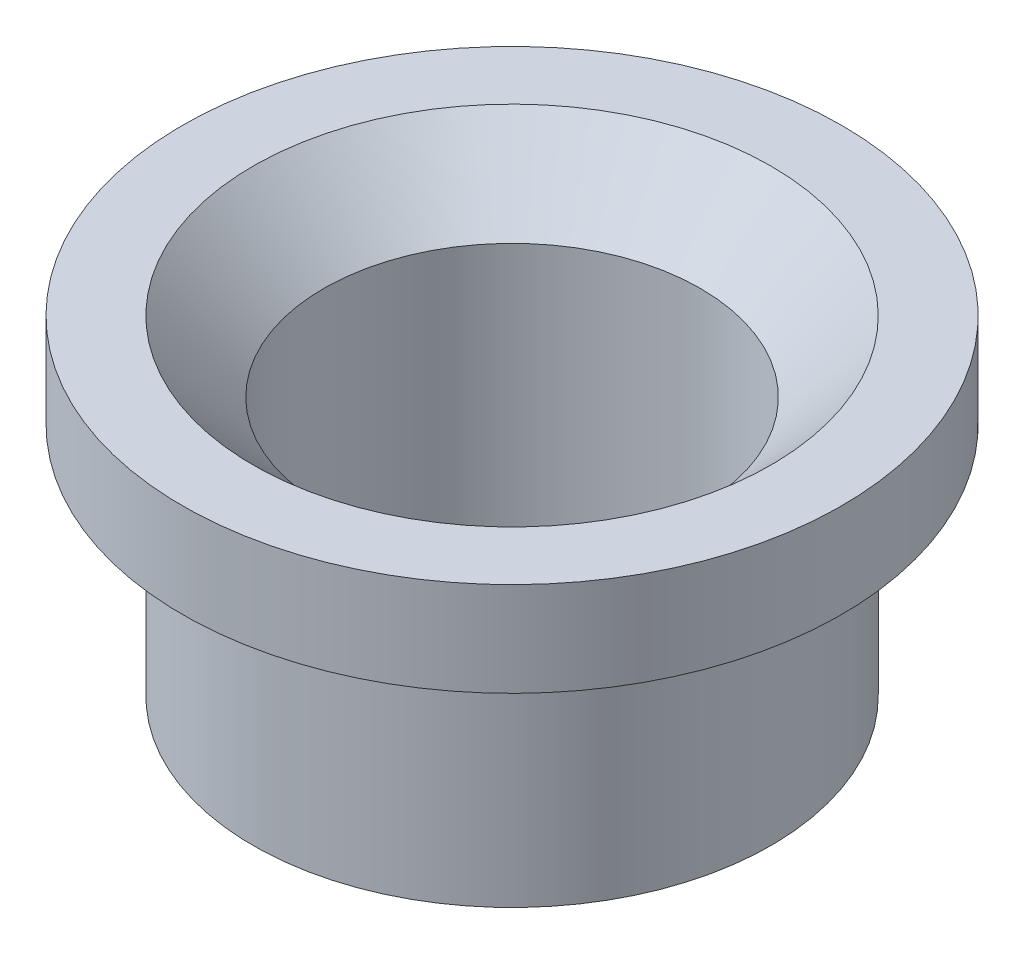
from build123d import *


with BuildPart() as part:
    # Bush Half-Section Profile → Flanged Bush Body (revolve)
    with BuildSketch(Plane.XY, mode=Mode.PRIVATE) as flanged_bush_body_sk:
        Polygon((12, 0), (12, 16.5), (16.5, 21), (21, 21), (21, 15), (16.5, 15), (16.5, 0), align=None)
    revolve(flanged_bush_body_sk.sketch.rotate(Axis((0, 0, 0), (0, 1, 0)), 90), axis=Axis((0, 0, 0), (0, 1, 0)))


solid = part.part
